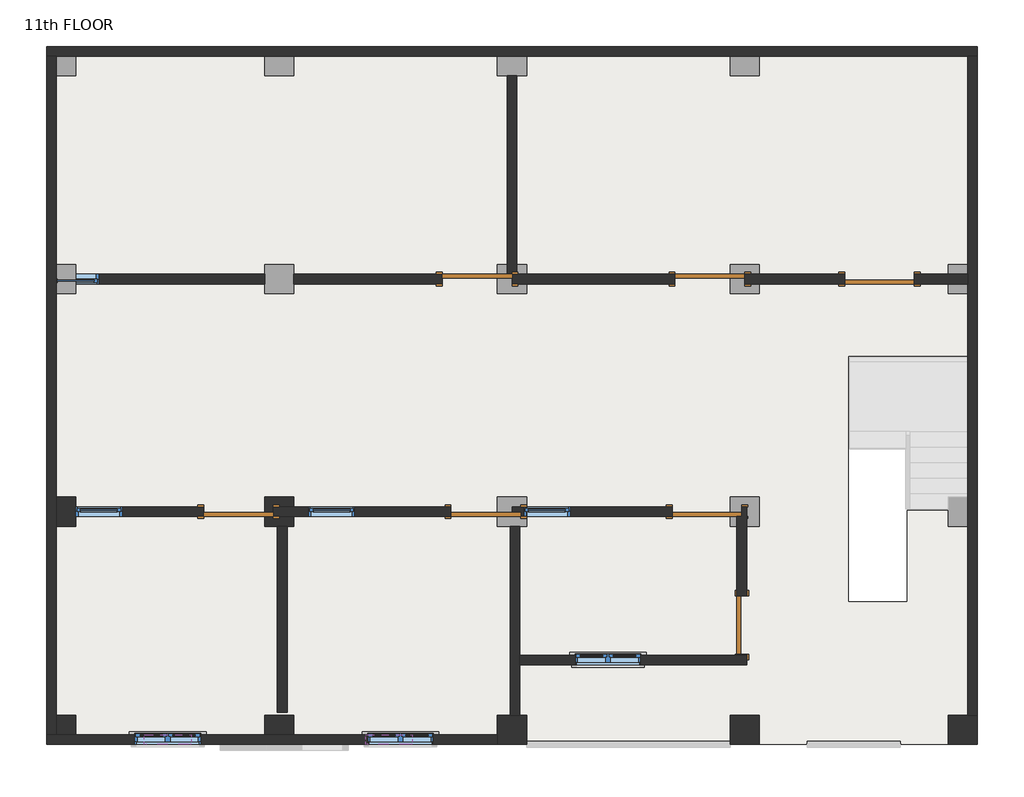
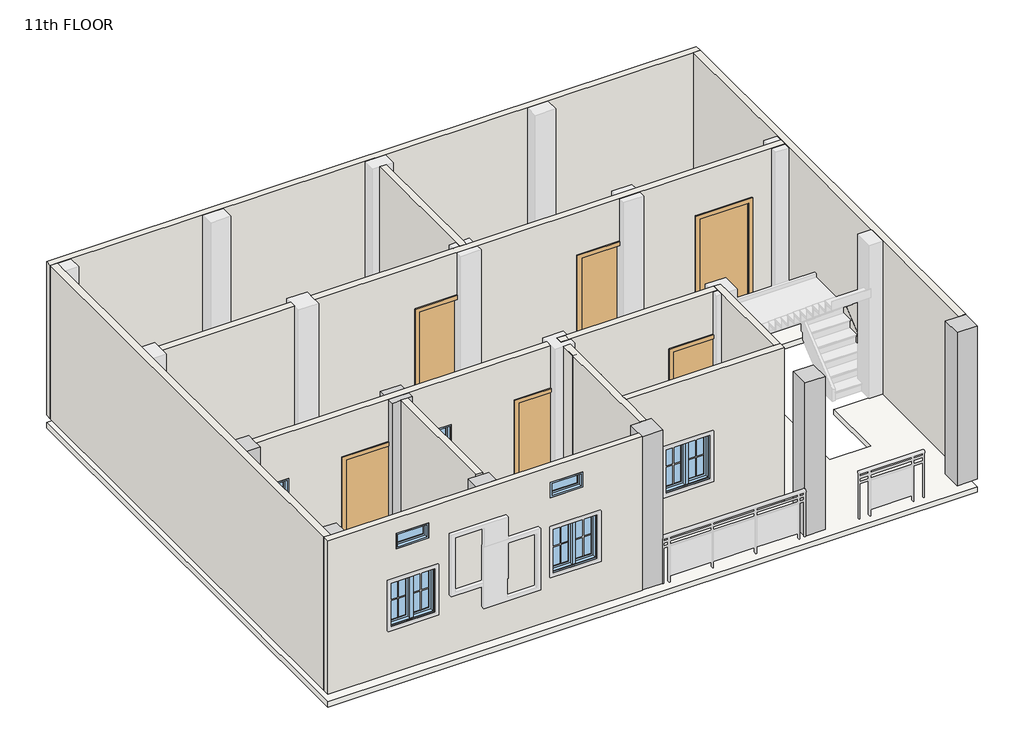
# One storey, part 1 of 2: 15 walls, 9 windows, 7 columns, 7 doors, 1 slab.
"""IFC4 building model written with IfcOpenShell, lengths in millimetres."""

from ifc_helpers import new_model, si_unit, frame, origin, place, context, project, spatial, polyline, outline, extrude, faceted_brep, transform, mapped, element, save
from components import door_e00f436c, door_a1797ceb, window_4c2727af, window_0bf3737e, window_78893e6c, window_0d9958e7

model = new_model("IFC4")

# Units and contexts
model_context = context("Model", 3, world=origin())
ifc_project = project(units=[si_unit("LENGTHUNIT", "METRE", prefix="MILLI")], contexts=[model_context])

# Site, building, storey
site = spatial("IfcSite", under=ifc_project)
building = spatial("IfcBuilding", under=site)
storey = spatial("IfcBuildingStorey", under=building, Name="11th FLOOR", Elevation=33375.6)

# Columns
placement = place(None, origin())
element("IfcColumn", 1, ObjectType="column family : column family", at=placement, inside=storey, context=model_context, shape_type="Brep", body=[
    faceted_brep([(-12576.097125, 2486.2065522, 33380.6), (-12957.097125, 2486.2065522, 33380.6), (-12957.097125, 2867.2065522, 33380.6), (-12576.097125, 2867.2065522, 33380.6), (-12576.097125, 2740.2065522, 33380.6), (-12842.797125, 2740.2065522, 33380.6), (-12842.797125, 2613.2065522, 33380.6), (-12576.097125, 2613.2065522, 33380.6), (-12576.097125, 2486.2065522, 36418.6), (-12576.097125, 2613.2065522, 36418.6), (-12957.097125, 2486.2065522, 36418.6), (-12957.097125, 2613.2065522, 36418.6), (-12957.097125, 2613.2065522, 35509.2), (-12957.097125, 2740.2065522, 35509.2), (-12957.097125, 2740.2065522, 36418.6), (-12957.097125, 2867.2065522, 36418.6), (-12576.097125, 2867.2065522, 36418.6), (-12842.797125, 2613.2065522, 35509.2), (-12842.797125, 2740.2065522, 35509.2), (-12576.097125, 2740.2065522, 36418.6)], [[[0, 1, 2, 3, 4, 5, 6, 7]], [[8, 0, 7, 9]], [[1, 0, 8, 10]], [[2, 1, 10, 11, 12, 13, 14, 15]], [[3, 2, 15, 16]], [[10, 8, 9, 11]], [[6, 17, 12, 11, 9, 7]], [[13, 18, 5, 4, 19, 14]], [[3, 16, 19, 4]], [[16, 15, 14, 19]], [[17, 18, 13, 12]], [[18, 17, 6, 5]]]),
])
element("IfcColumn", 2, ObjectType="column family : column family", at=placement, inside=storey, context=model_context, shape_type="SweptSolid", body=[
    extrude(outline(polyline([(-15433.597125, 2867.2065522), (-15433.597125, 2486.2065522), (-15687.597125, 2486.2065522), (-15687.597125, 2867.2065522), (-15433.597125, 2867.2065522)])), frame((0.0, 0.0, 33380.6), z_axis=(0.0, 0.0, 1.0), x_axis=(1.0, 0.0, 0.0)), (0.0, 0.0, 1.0), 3038.0),
])
element("IfcColumn", 3, ObjectType="column family : column family", at=placement, inside=storey, context=model_context, shape_type="SweptSolid", body=[
    extrude(outline(polyline([(-15433.597125, 9.7065522), (-15433.597125, -244.2934478), (-15687.597125, -244.2934478), (-15687.597125, 9.7065522), (-15433.597125, 9.7065522)])), frame((0.0, 0.0, 33380.6), z_axis=(0.0, 0.0, 1.0), x_axis=(1.0, 0.0, 0.0)), (0.0, 0.0, 1.0), 3038.0),
])
element("IfcColumn", 4, ObjectType="column family : column family", at=placement, inside=storey, context=model_context, shape_type="SweptSolid", body=[
    extrude(outline(polyline([(-3622.597125, 9.7065522), (-3622.597125, -371.2934478), (-4003.597125, -371.2934478), (-4003.597125, 9.7065522), (-3622.597125, 9.7065522)])), frame((0.0, 0.0, 33380.6), z_axis=(0.0, 0.0, 1.0), x_axis=(1.0, 0.0, 0.0)), (0.0, 0.0, 1.0), 3038.0),
])
element("IfcColumn", 5, ObjectType="column family : column family", at=placement, inside=storey, context=model_context, shape_type="SweptSolid", body=[
    extrude(outline(polyline([(-6480.097125, 9.7065522), (-6480.097125, -371.2934478), (-6861.097125, -371.2934478), (-6861.097125, 9.7065522), (-6480.097125, 9.7065522)])), frame((0.0, 0.0, 33380.6), z_axis=(0.0, 0.0, 1.0), x_axis=(1.0, 0.0, 0.0)), (0.0, 0.0, 1.0), 3038.0),
])
element("IfcColumn", 6, ObjectType="column family : column family", at=placement, inside=storey, context=model_context, shape_type="SweptSolid", body=[
    extrude(outline(polyline([(-9528.097125, 9.7065522), (-9528.097125, -371.2934478), (-9909.097125, -371.2934478), (-9909.097125, 9.7065522), (-9528.097125, 9.7065522)])), frame((0.0, 0.0, 33380.6), z_axis=(0.0, 0.0, 1.0), x_axis=(1.0, 0.0, 0.0)), (0.0, 0.0, 1.0), 3038.0),
])
element("IfcColumn", 7, ObjectType="column family : column family", at=placement, inside=storey, context=model_context, shape_type="SweptSolid", body=[
    extrude(outline(polyline([(-12957.097125, 9.7065522), (-12576.097125, 9.7065522), (-12576.097125, -244.2934478), (-12957.097125, -244.2934478), (-12957.097125, 9.7065522)])), frame((0.0, 0.0, 33380.6), z_axis=(0.0, 0.0, 1.0), x_axis=(1.0, 0.0, 0.0)), (0.0, 0.0, 1.0), 3038.0),
])

# Doors
door_shape = door_e00f436c(model_context)
element("IfcDoor", 8, ObjectType="Single-Flush : 30\" x 80\"", at=placement, inside=storey, context=model_context, shape_type="MappedRepresentation", body=[
    mapped(door_shape, transform((-6708.697125, 1190.8065522, 33375.6), x_axis=(0.0, -1.0, 0.0), y_axis=(1.0, 0.0, 0.0), z_axis=(0.0, 0.0, 1.0))),
])
door_2_shape = door_a1797ceb(model_context)
element("IfcDoor", 9, ObjectType="Single-Flush : 36\" x 84\"", at=placement, inside=storey, context=model_context, shape_type="MappedRepresentation", body=[
    mapped(door_2_shape, transform((-10175.797125, 5724.7065522, 33375.6), x_axis=(1.0, 0.0, 0.0), y_axis=(0.0, 1.0, 0.0), z_axis=(0.0, 0.0, 1.0))),
])
element("IfcDoor", 10, ObjectType="Single-Flush : 36\" x 84\"", at=placement, inside=storey, context=model_context, shape_type="MappedRepresentation", body=[
    mapped(door_2_shape, transform((-10061.497125, 2676.7065522, 33375.6), x_axis=(-1.0, 0.0, 0.0), y_axis=(0.0, -1.0, 0.0), z_axis=(0.0, 0.0, 1.0))),
])
element("IfcDoor", 11, ObjectType="Single-Flush : 36\" x 84\"", at=placement, inside=storey, context=model_context, shape_type="MappedRepresentation", body=[
    mapped(door_2_shape, transform((-13299.997125, 2676.7065522, 33375.6), x_axis=(-1.0, 0.0, 0.0), y_axis=(0.0, -1.0, 0.0), z_axis=(0.0, 0.0, 1.0))),
])
element("IfcDoor", 12, ObjectType="Single-Flush : 36\" x 84\"", at=placement, inside=storey, context=model_context, shape_type="MappedRepresentation", body=[
    mapped(door_2_shape, transform((-7127.797125, 5724.7065522, 33375.6), x_axis=(1.0, 0.0, 0.0), y_axis=(0.0, 1.0, 0.0), z_axis=(0.0, 0.0, 1.0))),
])
element("IfcDoor", 13, ObjectType="Single-Flush : 36\" x 84\"", at=placement, inside=storey, context=model_context, shape_type="MappedRepresentation", body=[
    mapped(door_2_shape, transform((-7165.897125, 2676.7065522, 33375.6), x_axis=(-1.0, 0.0, 0.0), y_axis=(0.0, -1.0, 0.0), z_axis=(0.0, 0.0, 1.0))),
])
element("IfcDoor", 14, ObjectType="Single-Flush : 36\" x 84\"", at=placement, inside=storey, context=model_context, shape_type="MappedRepresentation", body=[
    mapped(door_2_shape, transform((-4905.297125, 5724.7065522, 33375.6), x_axis=(-1.0, 0.0, 0.0), y_axis=(0.0, -1.0, 0.0), z_axis=(0.0, 0.0, 1.0))),
])

# Slab
element("IfcSlab", 15, ObjectType="Generic - 4\"", at=placement, inside=storey, context=model_context, shape_type="SweptSolid", body=[
    extrude(outline(polyline([(-3622.597125, 8772.7065522), (-3622.597125, -371.2934478), (-15814.597125, -371.2934478), (-15814.597125, 8772.7065522), (-3622.597125, 8772.7065522)]), holes=[polyline([(-3734.357125, 4711.0719226), (-5310.2646464, 4711.0719226), (-5310.2646464, 1502.3126957), (-4547.7736682, 1502.3126957), (-4547.7736682, 2699.911213), (-3734.357125, 2699.911213), (-3734.357125, 4711.0719226)])]), frame((0.0, 0.0, 33121.6), z_axis=(0.0, 0.0, 1.0), x_axis=(1.0, 0.0, 0.0)), (0.0, 0.0, 1.0), 101.6),
])

# Walls
element("IfcWall", 16, ObjectType="Generic - 5\"", at=placement, inside=storey, context=model_context, shape_type="Brep", body=[
    faceted_brep([(-15814.597125, 8645.7065522, 33375.6), (-15687.597125, 8645.7065522, 33375.6), (-3749.597125, 8645.7065522, 33375.6), (-3622.597125, 8645.7065522, 33375.6), (-3622.597125, 8645.7065522, 36423.6), (-3749.597125, 8645.7065522, 36423.6), (-15687.597125, 8645.7065522, 36423.6), (-15814.597125, 8645.7065522, 36423.6), (-15814.597125, 8772.7065522, 33375.6), (-15814.597125, 8772.7065522, 36423.6), (-3622.597125, 8772.7065522, 36423.6), (-3622.597125, 8772.7065522, 33375.6)], [[[0, 1, 2, 3, 4, 5, 6, 7]], [[8, 9, 10, 11]], [[3, 2, 1, 0, 8, 11]], [[7, 6, 5, 4, 10, 9]], [[4, 3, 11, 10]], [[0, 7, 9, 8]]]),
])
element("IfcWall", 17, ObjectType="Generic - 5\"", at=placement, inside=storey, context=model_context, shape_type="Brep", body=[
    faceted_brep([(-3749.597125, 8645.7065522, 33375.6), (-3749.597125, 5788.2065522, 33375.6), (-3749.597125, 5661.2065522, 33375.6), (-3749.597125, 9.7065522, 33375.6), (-3749.597125, 9.7065522, 36423.6), (-3749.597125, 5661.2065522, 36423.6), (-3749.597125, 5788.2065522, 36423.6), (-3749.597125, 8645.7065522, 36423.6), (-3622.597125, 8645.7065522, 33375.6), (-3622.597125, 8645.7065522, 36423.6), (-3622.597125, 9.7065522, 36423.6), (-3622.597125, 9.7065522, 36418.6), (-3622.597125, 9.7065522, 33380.6), (-3622.597125, 9.7065522, 33375.6)], [[[0, 1, 2, 3, 4, 5, 6, 7]], [[8, 9, 10, 11, 12, 13]], [[3, 2, 1, 0, 8, 13]], [[4, 3, 13, 12, 11, 10]], [[7, 6, 5, 4, 10, 9]], [[0, 7, 9, 8]]]),
])
element("IfcWall", 18, ObjectType="Generic - 5\"", at=placement, inside=storey, context=model_context, shape_type="Brep", body=[
    faceted_brep([(-9909.097125, -244.2934478, 33375.6), (-15687.597125, -244.2934478, 33375.6), (-15814.597125, -244.2934478, 33375.6), (-15814.597125, -244.2934478, 36423.6), (-15687.597125, -244.2934478, 36423.6), (-9909.097125, -244.2934478, 36423.6), (-13795.297125, -244.2934478, 35204.4), (-14658.897125, -244.2934478, 35204.4), (-14658.897125, -244.2934478, 34290.0), (-13795.297125, -244.2934478, 34290.0), (-10747.297125, -244.2934478, 35204.4), (-11610.897125, -244.2934478, 35204.4), (-11610.897125, -244.2934478, 34290.0), (-10747.297125, -244.2934478, 34290.0), (-13922.297125, -244.2934478, 36118.8), (-14531.897125, -244.2934478, 36118.8), (-14531.897125, -244.2934478, 35814.0), (-13922.297125, -244.2934478, 35814.0), (-11026.697125, -244.2934478, 36118.8), (-11636.297125, -244.2934478, 36118.8), (-11636.297125, -244.2934478, 35814.0), (-11026.697125, -244.2934478, 35814.0), (-9909.097125, -371.2934478, 33375.6), (-9909.097125, -371.2934478, 33380.6), (-9909.097125, -371.2934478, 36418.6), (-9909.097125, -371.2934478, 36423.6), (-15814.597125, -371.2934478, 36423.6), (-15814.597125, -371.2934478, 33375.6), (-13795.297125, -371.2934478, 35204.4), (-13795.297125, -371.2934478, 34290.0), (-14658.897125, -371.2934478, 34290.0), (-14658.897125, -371.2934478, 35204.4), (-10747.297125, -371.2934478, 35204.4), (-10747.297125, -371.2934478, 34290.0), (-11610.897125, -371.2934478, 34290.0), (-11610.897125, -371.2934478, 35204.4), (-13922.297125, -371.2934478, 36118.8), (-13922.297125, -371.2934478, 35814.0), (-14531.897125, -371.2934478, 35814.0), (-14531.897125, -371.2934478, 36118.8), (-11026.697125, -371.2934478, 36118.8), (-11026.697125, -371.2934478, 35814.0), (-11636.297125, -371.2934478, 35814.0), (-11636.297125, -371.2934478, 36118.8)], [[[0, 1, 2, 3, 4, 5], [6, 7, 8, 9], [10, 11, 12, 13], [14, 15, 16, 17], [18, 19, 20, 21]], [[22, 23, 24, 25, 26, 27], [28, 29, 30, 31], [32, 33, 34, 35], [36, 37, 38, 39], [40, 41, 42, 43]], [[2, 1, 0, 22, 27]], [[5, 4, 3, 26, 25]], [[0, 5, 25, 24, 23, 22]], [[3, 2, 27, 26]], [[29, 28, 6, 9]], [[30, 29, 9, 8]], [[31, 30, 8, 7]], [[28, 31, 7, 6]], [[33, 32, 10, 13]], [[34, 33, 13, 12]], [[35, 34, 12, 11]], [[32, 35, 11, 10]], [[37, 36, 14, 17]], [[38, 37, 17, 16]], [[39, 38, 16, 15]], [[36, 39, 15, 14]], [[41, 40, 18, 21]], [[42, 41, 21, 20]], [[43, 42, 20, 19]], [[40, 43, 19, 18]]]),
])
element("IfcWall", 19, ObjectType="Generic - 5\"", at=placement, inside=storey, context=model_context, shape_type="Brep", body=[
    faceted_brep([(-15687.597125, -244.2934478, 33375.6), (-15687.597125, 8645.7065522, 33375.6), (-15687.597125, 8645.7065522, 33380.6), (-15687.597125, 8645.7065522, 36418.6), (-15687.597125, 8645.7065522, 36423.6), (-15687.597125, -244.2934478, 36423.6), (-15687.597125, -244.2934478, 36418.6), (-15687.597125, -244.2934478, 33380.6), (-15814.597125, -244.2934478, 33375.6), (-15814.597125, -244.2934478, 36423.6), (-15814.597125, 8645.7065522, 36423.6), (-15814.597125, 8645.7065522, 33375.6)], [[[0, 1, 2, 3, 4, 5, 6, 7]], [[8, 9, 10, 11]], [[1, 0, 8, 11]], [[5, 4, 10, 9]], [[4, 3, 2, 1, 11, 10]], [[0, 7, 6, 5, 9, 8]]]),
])
element("IfcWall", 20, ObjectType="Generic - 5\"", at=placement, inside=storey, context=model_context, shape_type="SweptSolid", body=[
    extrude(outline(polyline([(33375.6, -15433.597125), (33375.6, -12957.097125), (36423.6, -12957.097125), (36423.6, -15433.597125), (35509.2, -15433.597125), (35509.2, -15128.797125), (33680.4, -15128.797125), (33680.4, -15433.597125), (33375.6, -15433.597125)])), frame((0.0, 5661.2065522, 0.0), z_axis=(0.0, 1.0, 0.0), x_axis=(0.0, 0.0, 1.0)), (0.0, 0.0, 1.0), 127.0),
])
element("IfcWall", 21, ObjectType="Generic - 5\"", at=placement, inside=storey, context=model_context, shape_type="Brep", body=[
    faceted_brep([(-9782.097125, 8391.7065522, 33375.6), (-9782.097125, 5788.2065522, 33375.6), (-9782.097125, 5788.2065522, 33380.6), (-9782.097125, 5788.2065522, 35509.2), (-9782.097125, 5788.2065522, 36418.6), (-9782.097125, 5788.2065522, 36423.6), (-9782.097125, 8391.7065522, 36423.6), (-9655.097125, 8391.7065522, 33375.6), (-9655.097125, 8391.7065522, 36423.6), (-9655.097125, 5788.2065522, 36423.6), (-9655.097125, 5788.2065522, 36418.6), (-9655.097125, 5788.2065522, 33380.6), (-9655.097125, 5788.2065522, 33375.6), (-9718.597125, 5788.2065522, 33375.6)], [[[0, 1, 2, 3, 4, 5, 6]], [[7, 8, 9, 10, 11, 12]], [[1, 0, 7, 12, 13]], [[6, 5, 9, 8]], [[0, 6, 8, 7]], [[5, 4, 3, 2, 1, 13, 12, 11, 10, 9]]]),
])
element("IfcWall", 22, ObjectType="Generic - 5\"", at=placement, inside=storey, context=model_context, shape_type="Brep", body=[
    faceted_brep([(-6670.597125, 5661.2065522, 33375.6), (-5362.497125, 5661.2065522, 33375.6), (-5362.497125, 5661.2065522, 35509.2), (-4448.097125, 5661.2065522, 35509.2), (-4448.097125, 5661.2065522, 33375.6), (-3749.597125, 5661.2065522, 33375.6), (-3749.597125, 5661.2065522, 33380.6), (-3749.597125, 5661.2065522, 36418.6), (-3749.597125, 5661.2065522, 36423.6), (-12576.097125, 5661.2065522, 36423.6), (-12576.097125, 5661.2065522, 33375.6), (-10632.997125, 5661.2065522, 33375.6), (-10632.997125, 5661.2065522, 35509.2), (-9909.097125, 5661.2065522, 35509.2), (-9718.597125, 5661.2065522, 35509.2), (-9718.597125, 5661.2065522, 33380.6), (-9718.597125, 5661.2065522, 33375.6), (-7584.997125, 5661.2065522, 33375.6), (-7584.997125, 5661.2065522, 35509.2), (-6861.097125, 5661.2065522, 35509.2), (-6670.597125, 5661.2065522, 35509.2), (-6670.597125, 5661.2065522, 33380.6), (-5362.497125, 5788.2065522, 35509.2), (-5362.497125, 5788.2065522, 33375.6), (-6670.597125, 5788.2065522, 33375.6), (-6670.597125, 5788.2065522, 33380.6), (-6670.597125, 5788.2065522, 35509.2), (-6861.097125, 5788.2065522, 35509.2), (-7584.997125, 5788.2065522, 35509.2), (-7584.997125, 5788.2065522, 33375.6), (-9655.097125, 5788.2065522, 33375.6), (-9718.597125, 5788.2065522, 33375.6), (-9718.597125, 5788.2065522, 33380.6), (-9718.597125, 5788.2065522, 35509.2), (-9782.097125, 5788.2065522, 35509.2), (-9909.097125, 5788.2065522, 35509.2), (-10632.997125, 5788.2065522, 35509.2), (-10632.997125, 5788.2065522, 33375.6), (-12576.097125, 5788.2065522, 33375.6), (-12576.097125, 5788.2065522, 36423.6), (-9782.097125, 5788.2065522, 36423.6), (-9655.097125, 5788.2065522, 36423.6), (-3749.597125, 5788.2065522, 36423.6), (-3749.597125, 5788.2065522, 36418.6), (-3749.597125, 5788.2065522, 33380.6), (-3749.597125, 5788.2065522, 33375.6), (-4448.097125, 5788.2065522, 33375.6), (-4448.097125, 5788.2065522, 35509.2)], [[[0, 1, 2, 3, 4, 5, 6, 7, 8, 9, 10, 11, 12, 13, 14, 15, 16, 17, 18, 19, 20, 21]], [[22, 23, 24, 25, 26, 27, 28, 29, 30, 31, 32, 33, 34, 35, 36, 37, 38, 39, 40, 41, 42, 43, 44, 45, 46, 47]], [[11, 10, 38, 37]], [[17, 16, 31, 30, 29]], [[46, 45, 5, 4]], [[24, 23, 1, 0]], [[9, 8, 42, 41, 40, 39]], [[10, 9, 39, 38]], [[8, 7, 6, 5, 45, 44, 43, 42]], [[33, 32, 31, 16, 15, 14]], [[36, 35, 34, 33, 14, 13, 12]], [[37, 36, 12, 11]], [[26, 25, 24, 0, 21, 20]], [[28, 27, 26, 20, 19, 18]], [[29, 28, 18, 17]], [[2, 1, 23, 22]], [[3, 2, 22, 47]], [[4, 3, 47, 46]]]),
])
element("IfcWall", 23, ObjectType="Generic - 5\"", at=placement, inside=storey, context=model_context, shape_type="Brep", body=[
    faceted_brep([(-14823.997125, 2613.2065522, 33680.4), (-15433.597125, 2613.2065522, 33680.4), (-15433.597125, 2613.2065522, 33375.6), (-13757.197125, 2613.2065522, 33375.6), (-13757.197125, 2613.2065522, 35509.2), (-12957.097125, 2613.2065522, 35509.2), (-12842.797125, 2613.2065522, 35509.2), (-12842.797125, 2613.2065522, 33380.6), (-12842.797125, 2613.2065522, 33375.6), (-10518.697125, 2613.2065522, 33375.6), (-10518.697125, 2613.2065522, 35509.2), (-9909.097125, 2613.2065522, 35509.2), (-9909.097125, 2613.2065522, 36423.6), (-15433.597125, 2613.2065522, 36423.6), (-15433.597125, 2613.2065522, 35509.2), (-14823.997125, 2613.2065522, 35509.2), (-12385.597125, 2613.2065522, 35509.2), (-11775.997125, 2613.2065522, 35509.2), (-11775.997125, 2613.2065522, 33680.4), (-12385.597125, 2613.2065522, 33680.4), (-15433.597125, 2740.2065522, 33375.6), (-15433.597125, 2740.2065522, 33680.4), (-14823.997125, 2740.2065522, 33680.4), (-14823.997125, 2740.2065522, 35509.2), (-15433.597125, 2740.2065522, 35509.2), (-15433.597125, 2740.2065522, 36423.6), (-9909.097125, 2740.2065522, 36423.6), (-9909.097125, 2740.2065522, 35509.2), (-10518.697125, 2740.2065522, 35509.2), (-10518.697125, 2740.2065522, 33375.6), (-12842.797125, 2740.2065522, 33375.6), (-12842.797125, 2740.2065522, 33380.6), (-12842.797125, 2740.2065522, 35509.2), (-12957.097125, 2740.2065522, 35509.2), (-13757.197125, 2740.2065522, 35509.2), (-13757.197125, 2740.2065522, 33375.6), (-12385.597125, 2740.2065522, 35509.2), (-12385.597125, 2740.2065522, 33680.4), (-11775.997125, 2740.2065522, 33680.4), (-11775.997125, 2740.2065522, 35509.2)], [[[0, 1, 2, 3, 4, 5, 6, 7, 8, 9, 10, 11, 12, 13, 14, 15], [16, 17, 18, 19]], [[20, 21, 22, 23, 24, 25, 26, 27, 28, 29, 30, 31, 32, 33, 34, 35], [36, 37, 38, 39]], [[30, 29, 9, 8]], [[20, 35, 3, 2]], [[26, 12, 11, 27]], [[13, 12, 26, 25]], [[14, 13, 25, 24]], [[2, 1, 21, 20]], [[28, 10, 9, 29]], [[10, 28, 27, 11]], [[4, 3, 35, 34]], [[6, 5, 4, 34, 33, 32]], [[8, 7, 6, 32, 31, 30]], [[22, 21, 1, 0]], [[23, 22, 0, 15]], [[24, 23, 15, 14]], [[37, 36, 16, 19]], [[38, 37, 19, 18]], [[39, 38, 18, 17]], [[36, 39, 17, 16]]]),
])
element("IfcWall", 24, ObjectType="Generic - 5\"", at=placement, inside=storey, context=model_context, shape_type="Brep", body=[
    faceted_brep([(-9616.997125, 9.7065522, 33375.6), (-9616.997125, 670.1065522, 33375.6), (-9616.997125, 797.1065522, 33375.6), (-9616.997125, 2486.2065522, 33375.6), (-9616.997125, 2486.2065522, 36423.6), (-9616.997125, 797.1065522, 36423.6), (-9616.997125, 670.1065522, 36423.6), (-9616.997125, 9.7065522, 36423.6), (-9743.997125, 9.7065522, 33375.6), (-9743.997125, 9.7065522, 36423.6), (-9743.997125, 2486.2065522, 36423.6), (-9743.997125, 2486.2065522, 33375.6)], [[[0, 1, 2, 3, 4, 5, 6, 7]], [[8, 9, 10, 11]], [[3, 2, 1, 0, 8, 11]], [[4, 3, 11, 10]], [[7, 6, 5, 4, 10, 9]], [[0, 7, 9, 8]]]),
])
element("IfcWall", 25, ObjectType="Generic - 5\"", at=placement, inside=storey, context=model_context, shape_type="SweptSolid", body=[
    extrude(outline(polyline([(-9743.997125, 2181.4065522), (-9743.997125, 2486.2065522), (-9616.997125, 2486.2065522), (-9616.997125, 2181.4065522), (-9743.997125, 2181.4065522)])), frame((0.0, 0.0, 33375.6), z_axis=(0.0, 0.0, 1.0), x_axis=(1.0, 0.0, 0.0)), (0.0, 0.0, 1.0), 3048.0),
])
element("IfcWall", 26, ObjectType="Generic - 5\"", at=placement, inside=storey, context=model_context, shape_type="Brep", body=[
    faceted_brep([(-6772.197125, 2613.2065522, 36423.6), (-9718.597125, 2613.2065522, 36423.6), (-9718.597125, 2613.2065522, 36418.6), (-9718.597125, 2613.2065522, 33380.6), (-9718.597125, 2613.2065522, 33375.6), (-7623.097125, 2613.2065522, 33375.6), (-7623.097125, 2613.2065522, 35509.2), (-6861.097125, 2613.2065522, 35509.2), (-6772.197125, 2613.2065522, 35509.2), (-6772.197125, 2613.2065522, 36418.6), (-9566.197125, 2613.2065522, 35509.2), (-9528.097125, 2613.2065522, 35509.2), (-8956.597125, 2613.2065522, 35509.2), (-8956.597125, 2613.2065522, 33680.4), (-9528.097125, 2613.2065522, 33680.4), (-9566.197125, 2613.2065522, 33680.4), (-9718.597125, 2740.2065522, 36423.6), (-6772.197125, 2740.2065522, 36423.6), (-6772.197125, 2740.2065522, 35509.2), (-6861.097125, 2740.2065522, 35509.2), (-7623.097125, 2740.2065522, 35509.2), (-7623.097125, 2740.2065522, 33375.6), (-9718.597125, 2740.2065522, 33375.6), (-9718.597125, 2740.2065522, 33380.6), (-9718.597125, 2740.2065522, 36418.6), (-9566.197125, 2740.2065522, 35509.2), (-9566.197125, 2740.2065522, 33680.4), (-9528.097125, 2740.2065522, 33680.4), (-8956.597125, 2740.2065522, 33680.4), (-8956.597125, 2740.2065522, 35509.2), (-9528.097125, 2740.2065522, 35509.2)], [[[0, 1, 2, 3, 4, 5, 6, 7, 8, 9], [10, 11, 12, 13, 14, 15]], [[16, 17, 18, 19, 20, 21, 22, 23, 24], [25, 26, 27, 28, 29, 30]], [[4, 22, 21, 5]], [[1, 0, 17, 16]], [[4, 3, 2, 1, 16, 24, 23, 22]], [[26, 25, 10, 15]], [[28, 27, 26, 15, 14, 13]], [[29, 28, 13, 12]], [[25, 30, 29, 12, 11, 10]], [[20, 6, 5, 21]], [[6, 20, 19, 18, 8, 7]], [[17, 0, 9, 8, 18]]]),
])
element("IfcWall", 27, ObjectType="Generic - 5\"", at=placement, inside=storey, context=model_context, shape_type="Brep", body=[
    faceted_brep([(-6645.197125, 797.1065522, 33375.6), (-6645.197125, 809.8065522, 33375.6), (-6645.197125, 809.8065522, 35407.6), (-6645.197125, 1571.8065522, 35407.6), (-6645.197125, 1571.8065522, 33375.6), (-6645.197125, 2740.2065522, 33375.6), (-6645.197125, 2740.2065522, 33380.6), (-6645.197125, 2740.2065522, 36418.6), (-6645.197125, 2740.2065522, 36423.6), (-6645.197125, 797.1065522, 36423.6), (-6772.197125, 809.8065522, 35407.6), (-6772.197125, 809.8065522, 33375.6), (-6772.197125, 797.1065522, 33375.6), (-6772.197125, 797.1065522, 36423.6), (-6772.197125, 2613.2065522, 36423.6), (-6772.197125, 2740.2065522, 36423.6), (-6772.197125, 2740.2065522, 35509.2), (-6772.197125, 2613.2065522, 35509.2), (-6772.197125, 2613.2065522, 33380.6), (-6772.197125, 2613.2065522, 33375.6), (-6772.197125, 1571.8065522, 33375.6), (-6772.197125, 1571.8065522, 35407.6), (-6708.697125, 2613.2065522, 33375.6), (-6708.697125, 2740.2065522, 33375.6), (-6708.697125, 2613.2065522, 35509.2), (-6708.697125, 2613.2065522, 33380.6), (-6708.697125, 2740.2065522, 35509.2), (-6708.697125, 2740.2065522, 33380.6)], [[[0, 1, 2, 3, 4, 5, 6, 7, 8, 9]], [[10, 11, 12, 13, 14, 15, 16, 17, 18, 19, 20, 21]], [[20, 19, 22, 23, 5, 4]], [[12, 11, 1, 0]], [[9, 8, 15, 14, 13]], [[24, 25, 22, 19, 18, 17]], [[26, 24, 17, 16]], [[22, 25, 24, 26, 27, 23]], [[8, 7, 6, 5, 23, 27, 26, 16, 15]], [[0, 9, 13, 12]], [[2, 1, 11, 10]], [[3, 2, 10, 21]], [[4, 3, 21, 20]]]),
])
element("IfcWall", 28, ObjectType="Generic - 5\"", at=placement, inside=storey, context=model_context, shape_type="Brep", body=[
    faceted_brep([(-9718.597125, 2613.2065522, 33375.6), (-9566.197125, 2613.2065522, 33375.6), (-9566.197125, 2613.2065522, 33680.4), (-9566.197125, 2613.2065522, 35509.2), (-9566.197125, 2613.2065522, 36423.6), (-9718.597125, 2613.2065522, 36423.6), (-9718.597125, 2613.2065522, 36418.6), (-9718.597125, 2613.2065522, 33380.6), (-9718.597125, 2740.2065522, 33375.6), (-9718.597125, 2740.2065522, 33380.6), (-9718.597125, 2740.2065522, 36418.6), (-9718.597125, 2740.2065522, 36423.6), (-9566.197125, 2740.2065522, 36423.6), (-9566.197125, 2740.2065522, 35509.2), (-9566.197125, 2740.2065522, 33680.4), (-9566.197125, 2740.2065522, 33375.6)], [[[0, 1, 2, 3, 4, 5, 6, 7]], [[8, 9, 10, 11, 12, 13, 14, 15]], [[1, 0, 8, 15]], [[4, 3, 2, 1, 15, 14, 13, 12]], [[5, 4, 12, 11]], [[0, 7, 6, 5, 11, 10, 9, 8]]]),
])
element("IfcWall", 29, ObjectType="Generic - 5\"", at=placement, inside=storey, context=model_context, shape_type="SweptSolid", body=[
    extrude(outline(polyline([(-12791.997125, 47.8065522), (-12791.997125, 2486.2065522), (-12664.997125, 2486.2065522), (-12664.997125, 47.8065522), (-12791.997125, 47.8065522)])), frame((0.0, 0.0, 33375.6), z_axis=(0.0, 0.0, 1.0), x_axis=(1.0, 0.0, 0.0)), (0.0, 0.0, 1.0), 3048.0),
])
element("IfcWall", 30, ObjectType="Generic - 5\"", at=placement, inside=storey, context=model_context, shape_type="Brep", body=[
    faceted_brep([(-9616.997125, 670.1065522, 33375.6), (-6645.197125, 670.1065522, 33375.6), (-6645.197125, 670.1065522, 36423.6), (-9616.997125, 670.1065522, 36423.6), (-8029.497125, 670.1065522, 35204.4), (-8029.497125, 670.1065522, 34290.0), (-8893.097125, 670.1065522, 34290.0), (-8893.097125, 670.1065522, 35204.4), (-9616.997125, 797.1065522, 33375.6), (-9616.997125, 797.1065522, 36423.6), (-6772.197125, 797.1065522, 36423.6), (-6645.197125, 797.1065522, 36423.6), (-6645.197125, 797.1065522, 33375.6), (-6772.197125, 797.1065522, 33375.6), (-8029.497125, 797.1065522, 35204.4), (-8893.097125, 797.1065522, 35204.4), (-8893.097125, 797.1065522, 34290.0), (-8029.497125, 797.1065522, 34290.0)], [[[0, 1, 2, 3], [4, 5, 6, 7]], [[8, 9, 10, 11, 12, 13], [14, 15, 16, 17]], [[1, 0, 8, 13, 12]], [[3, 2, 11, 10, 9]], [[0, 3, 9, 8]], [[2, 1, 12, 11]], [[5, 4, 14, 17]], [[6, 5, 17, 16]], [[7, 6, 16, 15]], [[4, 7, 15, 14]]]),
])

# Windows
window_shape = window_4c2727af(model_context)
element("IfcWindow", 31, ObjectType="Fixed : 24\" x 12\"", at=placement, inside=storey, context=model_context, shape_type="MappedRepresentation", body=[
    mapped(window_shape, transform((-14188.997125, -307.7934478, 34899.6), x_axis=(1.0, 0.0, 0.0), y_axis=(0.0, 1.0, 0.0), z_axis=(0.0, 0.0, 1.0))),
])
element("IfcWindow", 32, ObjectType="Fixed : 24\" x 12\"", at=placement, inside=storey, context=model_context, shape_type="MappedRepresentation", body=[
    mapped(window_shape, transform((-11293.397125, -307.7934478, 34899.6), x_axis=(1.0, 0.0, 0.0), y_axis=(0.0, 1.0, 0.0), z_axis=(0.0, 0.0, 1.0))),
])
window_2_shape = window_0bf3737e(model_context)
element("IfcWindow", 33, ObjectType="Fixed : 24\" x 72\"", at=placement, inside=storey, context=model_context, shape_type="MappedRepresentation", body=[
    mapped(window_2_shape, transform((-15471.697125, 5724.7065522, 33375.6), x_axis=(-1.0, 0.0, 0.0), y_axis=(0.0, -1.0, 0.0), z_axis=(0.0, 0.0, 1.0))),
])
window_3_shape = window_78893e6c(model_context)
element("IfcWindow", 34, ObjectType="Fixed : 24\" x 72\"", at=placement, inside=storey, context=model_context, shape_type="MappedRepresentation", body=[
    mapped(window_3_shape, transform((-15166.897125, 2676.7065522, 33375.6), x_axis=(-1.0, 0.0, 0.0), y_axis=(0.0, -1.0, 0.0), z_axis=(0.0, 0.0, 1.0))),
])
element("IfcWindow", 35, ObjectType="Fixed : 24\" x 72\"", at=placement, inside=storey, context=model_context, shape_type="MappedRepresentation", body=[
    mapped(window_3_shape, transform((-12118.897125, 2676.7065522, 33375.6), x_axis=(-1.0, 0.0, 0.0), y_axis=(0.0, -1.0, 0.0), z_axis=(0.0, 0.0, 1.0))),
])
element("IfcWindow", 36, ObjectType="Fixed : 24\" x 72\"", at=placement, inside=storey, context=model_context, shape_type="MappedRepresentation", body=[
    mapped(window_3_shape, transform((-9299.497125, 2676.7065522, 33375.6), x_axis=(-1.0, 0.0, 0.0), y_axis=(0.0, -1.0, 0.0), z_axis=(0.0, 0.0, 1.0))),
])
window_4_shape = window_0d9958e7(model_context)
element("IfcWindow", 37, ObjectType="Window-Casement-Double : 34\" x 36\"", at=placement, inside=storey, context=model_context, shape_type="MappedRepresentation", body=[
    mapped(window_4_shape, transform((-14227.097125, -307.7934478, 33375.6), x_axis=(1.0, 0.0, 0.0), y_axis=(0.0, 1.0, 0.0), z_axis=(0.0, 0.0, 1.0))),
])
element("IfcWindow", 38, ObjectType="Window-Casement-Double : 34\" x 36\"", at=placement, inside=storey, context=model_context, shape_type="MappedRepresentation", body=[
    mapped(window_4_shape, transform((-11179.097125, -307.7934478, 33375.6), x_axis=(1.0, 0.0, 0.0), y_axis=(0.0, 1.0, 0.0), z_axis=(0.0, 0.0, 1.0))),
])
element("IfcWindow", 39, ObjectType="Window-Casement-Double : 34\" x 36\"", at=placement, inside=storey, context=model_context, shape_type="MappedRepresentation", body=[
    mapped(window_4_shape, transform((-8461.297125, 733.6065522, 33375.6), x_axis=(1.0, 0.0, 0.0), y_axis=(0.0, 1.0, 0.0), z_axis=(0.0, 0.0, 1.0))),
])

save(model, "model.ifc")

# Revit data of these elements
# Type "column family : column family"
#   w2 [instance default] = 0' - 9.88189"
#   w1 [instance default] = 0' - 9.01575"
#   Depth = 1' - 11.62205"
#   Width = 1' - 11.62205"
# Type "Single-Flush : 30\" x 80\""
#   Type Mark = "5"
#   Construction Type Id = "MDOOR"
#   Assembly Code = "C1020"
#   Analytic Construction = "Metal"
#   Thickness = 0' - 2"
#   Heat Transfer Coefficient (U) = 0.651978 BTU/(h·ft²·°F)
#   Height = 6' - 8"
#   Trim Projection Ext = 0' - 1"
#   Trim Projection Int = 0' - 1"
#   Trim Width = 0' - 3"
#   Width = 2' - 6"
#   Define Thermal Properties by = 1
#   Define Thermal Properties by = 1
#   Door Material = Door - Panel
#   Frame Material = Door - Frame
#   Visual Light Transmittance = 0
#   Solar Heat Gain Coefficient = 0
#   Function = (empty or 0)
#   Wall Closure = (empty or 0)
# Type "Single-Flush : 36\" x 84\""
#   Type Mark = "1"
#   Construction Type Id = "MDOOR"
#   Assembly Code = "C1020"
#   Analytic Construction = "Metal"
#   Thickness = 0' - 2"
#   Heat Transfer Coefficient (U) = 0.651978 BTU/(h·ft²·°F)
#   Height = 7' - 0"
#   Trim Projection Ext = 0' - 1"
#   Trim Projection Int = 0' - 1"
#   Trim Width = 0' - 3"
#   Width = 3' - 0"
#   Define Thermal Properties by = 1
#   Define Thermal Properties by = 1
#   Door Material = Door - Panel
#   Frame Material = Door - Frame
#   Visual Light Transmittance = 0
#   Solar Heat Gain Coefficient = 0
#   Function = (empty or 0)
#   Wall Closure = (empty or 0)
# Type "Generic - 4\""
#   Assembly Code = "B1010"
#   Function = 0
#   Layers, outside or top first: 0' - 4" no material (function 1)
# Type "Generic - 5\""
#   Assembly Code = "B2010"
#   Layers, outside or top first: 0' - 5" no material (function 1)
# Type "Fixed : 24\" x 12\""
#   Type Mark = "4"
#   Construction Type Id = "GSP4R"
#   Assembly Code = "B2020100"
#   Analytic Construction = "1/8 in Pilkington single glazing"
#   Visual Light Transmittance = 0.9
#   Solar Heat Gain Coefficient = 0.78
#   Heat Transfer Coefficient (U) = 0.6496 BTU/(h·ft²·°F)
#   Height = 1' - 0"
#   Default Sill Height = 3' - 0"
#   Width = 2' - 0"
#   Window Inset = 0' - 0 3/4"
#   Define Thermal Properties by = 1
#   Define Thermal Properties by = 1
#   Glass Pane Material = Glass
#   Sash Material = Sash
#   Wall Closure = (empty or 0)
# Type "Fixed : 24\" x 72\""
#   Type Mark = "7"
#   Construction Type Id = "GSP4R"
#   Assembly Code = "B2020100"
#   Analytic Construction = "1/8 in Pilkington single glazing"
#   Visual Light Transmittance = 0.9
#   Solar Heat Gain Coefficient = 0.78
#   Heat Transfer Coefficient (U) = 0.6496 BTU/(h·ft²·°F)
#   Height = 6' - 0"
#   Default Sill Height = 1' - 0"
#   Width = 2' - 0"
#   Window Inset = 0' - 0 3/4"
#   Define Thermal Properties by = 1
#   Define Thermal Properties by = 1
#   Glass Pane Material = Glass
#   Sash Material = Sash
#   Wall Closure = (empty or 0)
# Type "Window-Casement-Double : 34\" x 36\""
#   Type Mark = "14"
#   Fire Rating = "0.5h"
#   Assembly Code = "B2020100"
#   Analytic Construction = "Double glazing - domestic"
#   Frame Extension [instance default] = 0' - 0 1/4"
#   Window Inset [instance default] = 0' - 0"
#   Wall Thickness [instance default] = 0' - 6"
#   Interior Wall Closure [instance default] = 0' - 2 1/4"
#   Half Width = 1' - 5"
#   Visual Light Transmittance = 0.81
#   Thermal Resistance (R) = 1.8146 (h·ft²·°F)/BTU
#   Solar Heat Gain Coefficient = 0.76
#   Rough Width = 2' - 10 1/2"
#   Rough Height = 3' - 0 1/2"
#   Height = 3' - 0"
#   Heat Transfer Coefficient (U) = 0.5511 BTU/(h·ft²·°F)
#   Exterior Wall Closure [instance default] = 0' - 1 1/4"
#   Extension Jamb [instance default] = 0' - 2 1/4"
#   Default Sill Height = 3' - 0"
#   Width = 2' - 10"
#   Define Thermal Properties by = 0
#   Muntin Visibility = yes
#   Interior Trim Visibility [instance default] = yes
#   Exterior Trim Visibility [instance default] = yes
#   Extension Jamb Visibility [instance default] = yes
#   Interior Trim Material = Wood - Stained
#   Muntin Pattern = Muntin Pattern_2x2 : Muntin Pattern_2x2
#   Interior Trim = Trim-Window-Interior-Flat : Picture Frame
#   Interior Frame Material = Wood - Stained
#   Glass Panel Material = Glass
#   Exterior Trim Material = Clad - White
#   Exterior Trim = Trim-Window-Exterior-Flat : with Sill
#   Exterior Frame Material = Clad - White
#   Wall Closure = (empty or 0)
# Element 1 (IfcColumn, "column family : column family")
#   w2 = 1' - 3"
#   w1 = 1' - 3"
#   Phase Created = New Construction
#   Materials on its faces: "Default Wall", "inside wall"
# Element 2 (IfcColumn, "column family : column family")
#   w2 = 1' - 3"
#   w1 = 0' - 10"
#   Phase Created = New Construction
#   Materials on its faces: "inside wall", "Default Wall"
# Elements 3, 7 (IfcColumn, "column family : column family")
#   w2 = 1' - 3"
#   w1 = 1' - 3"
#   Phase Created = New Construction
#   Materials on its faces: "Default Wall"
# Element 4 (IfcColumn, "column family : column family")
#   w2 = 1' - 3"
#   w1 = 1' - 3"
#   Phase Created = New Construction
#   Materials on its faces: "Clad - White", "Default Wall"
# Element 5 (IfcColumn, "column family : column family")
#   w2 = 1' - 3"
#   w1 = 1' - 3"
#   Phase Created = New Construction
#   Materials on its faces: "out side wall"
# Element 6 (IfcColumn, "column family : column family")
#   w2 = 1' - 3"
#   w1 = 1' - 3"
#   Phase Created = New Construction
#   Materials on its faces: "out side wall", "Default Wall"
# Element 8 (IfcDoor, "Single-Flush : 30\" x 80\"")
#   Phase Created = New Construction
#   Materials on its faces: "Door - Frame", "Door - Panel"
# Elements 9, 10, 11, 12, 13, 14 (IfcDoor, "Single-Flush : 36\" x 84\"")
#   Phase Created = New Construction
#   Materials on its faces: "Door - Frame", "Door - Panel"
# Element 15 (IfcSlab, "Generic - 4\"")
#   Height Offset From Level = -0' - 6"
#   Phase Created = New Construction
#   Materials on its faces: "Default Floor", "Clad - White", "floor"
# Element 16 (IfcWall, "Generic - 5\"")
#   Top Offset = 0' - 0"
#   Base Offset = 0' - 0"
#   wall height = 10' - 0"
#   Phase Created = New Construction
#   Base Constraint = 11th FLOOR
#   Top Constraint = 12th FLOOR
#   Materials on its faces: "Default Wall", "Clad - White"
# Element 17 (IfcWall, "Generic - 5\"")
#   Top Offset = 0' - 0"
#   Base Offset = 0' - 0"
#   wall height = 10' - 0"
#   Phase Created = New Construction
#   Base Constraint = 11th FLOOR
#   Top Constraint = 12th FLOOR
#   Materials on its faces: "Default Wall", "grey", "Clad - White"
# Element 18 (IfcWall, "Generic - 5\"")
#   Top Offset = 0' - 0"
#   Base Offset = 0' - 0"
#   wall height = 10' - 0"
#   Phase Created = New Construction
#   Base Constraint = 11th FLOOR
#   Top Constraint = 12th FLOOR
#   Materials on its faces: "Default Wall", "out side wall", "Clad - White"
# Element 19 (IfcWall, "Generic - 5\"")
#   Top Offset = 0' - 0"
#   Base Offset = 0' - 0"
#   wall height = 10' - 0"
#   Phase Created = New Construction
#   Base Constraint = 11th FLOOR
#   Top Constraint = 12th FLOOR
#   Materials on its faces: "Default Wall", "inside wall", "Clad - White"
# Elements 20, 23, 26, 27 (IfcWall, "Generic - 5\"")
#   Top Offset = 0' - 0"
#   Base Offset = 0' - 0"
#   wall height = 10' - 0"
#   Phase Created = New Construction
#   Base Constraint = 11th FLOOR
#   Top Constraint = 12th FLOOR
#   Materials on its faces: "Default Wall", "inside wall"
# Elements 21, 25, 28, 29 (IfcWall, "Generic - 5\"")
#   Top Offset = 0' - 0"
#   Base Offset = 0' - 0"
#   wall height = 10' - 0"
#   Phase Created = New Construction
#   Base Constraint = 11th FLOOR
#   Top Constraint = 12th FLOOR
#   Materials on its faces: "Default Wall"
# Elements 22, 24 (IfcWall, "Generic - 5\"")
#   Top Offset = 0' - 0"
#   Base Offset = 0' - 0"
#   wall height = 10' - 0"
#   Phase Created = New Construction
#   Base Constraint = 11th FLOOR
#   Top Constraint = 12th FLOOR
#   Materials on its faces: "Default Wall", "grey"
# Element 30 (IfcWall, "Generic - 5\"")
#   Top Offset = 0' - 0"
#   Base Offset = 0' - 0"
#   wall height = 10' - 0"
#   Phase Created = New Construction
#   Base Constraint = 11th FLOOR
#   Top Constraint = 12th FLOOR
#   Materials on its faces: "Default Wall", "grey", "inside wall"
# Element 31 (IfcWindow, "Fixed : 24\" x 12\"")
#   Mark = "106"
#   Phase Created = New Construction
#   Materials on its faces: "Sash", "Glass"
# Element 32 (IfcWindow, "Fixed : 24\" x 12\"")
#   Mark = "107"
#   Phase Created = New Construction
#   Materials on its faces: "Sash", "Glass"
# Element 33 (IfcWindow, "Fixed : 24\" x 72\"")
#   Mark = "100"
#   Phase Created = New Construction
#   Materials on its faces: "Sash", "Glass"
# Element 34 (IfcWindow, "Fixed : 24\" x 72\"")
#   Mark = "101"
#   Phase Created = New Construction
#   Materials on its faces: "Sash", "Glass"
# Element 35 (IfcWindow, "Fixed : 24\" x 72\"")
#   Mark = "102"
#   Phase Created = New Construction
#   Materials on its faces: "Sash", "Glass"
# Element 36 (IfcWindow, "Fixed : 24\" x 72\"")
#   Mark = "103"
#   Phase Created = New Construction
#   Materials on its faces: "Sash", "Glass"
# Element 37 (IfcWindow, "Window-Casement-Double : 34\" x 36\"")
#   Mark = "104"
#   Window Inset = 0' - 0"
#   Interior Wall Closure = 0' - 2 1/4"
#   Frame Extension = 0' - 0 1/4"
#   Exterior Wall Closure = 0' - 1 1/4"
#   Interior Trim Visibility = yes
#   Exterior Trim Visibility = yes
#   Phase Created = New Construction
#   Materials on its faces: "Wood - Stained", "Glass", "Clad - White"
# Element 38 (IfcWindow, "Window-Casement-Double : 34\" x 36\"")
#   Mark = "105"
#   Window Inset = 0' - 0"
#   Interior Wall Closure = 0' - 2 1/4"
#   Frame Extension = 0' - 0 1/4"
#   Exterior Wall Closure = 0' - 1 1/4"
#   Interior Trim Visibility = yes
#   Exterior Trim Visibility = yes
#   Phase Created = New Construction
#   Materials on its faces: "Wood - Stained", "Glass", "Clad - White"
# Element 39 (IfcWindow, "Window-Casement-Double : 34\" x 36\"")
#   Mark = "108"
#   Window Inset = 0' - 0"
#   Interior Wall Closure = 0' - 2 1/4"
#   Frame Extension = 0' - 0 1/4"
#   Exterior Wall Closure = 0' - 1 1/4"
#   Interior Trim Visibility = yes
#   Exterior Trim Visibility = yes
#   Phase Created = New Construction
#   Materials on its faces: "Wood - Stained", "Glass", "Clad - White"
# Materials
#   "Door - Panel": class "Wood", colour RGB 210 159 95, transparency 0, Cost = 0
#   "Door - Frame": colour RGB 118 70 51, transparency 0, Cost = 0
#   "Glass": class "Glass", colour RGB 0 128 192, transparency 0.75, Description = "Soda Lime Glass", Cost = 0
#   "Sash": class "Wood", colour RGB 224 178 126, transparency 0, Cost = 0
#   "Wood - Stained": class "Wood", colour RGB 224 178 126, transparency 0, Cost = 0
#   "Clad - White": class "Wood", colour RGB 242 242 238, transparency 0, Cost = 0
#   "Default Wall": colour RGB 128 128 128, transparency 0, Cost = 0
#   "inside wall": class "Generic", colour RGB 199 224 95, transparency 0, Cost = 0
#   "out side wall": class "Generic", colour RGB 16 106 159, transparency 0, Cost = 0
#   "Default Floor": colour RGB 128 128 128, transparency 0, Cost = 0
#   "floor": class "Generic", colour RGB 255 255 255, transparency 0, Cost = 0
#   "grey": class "Generic", colour RGB 80 80 80, transparency 0, Cost = 0
